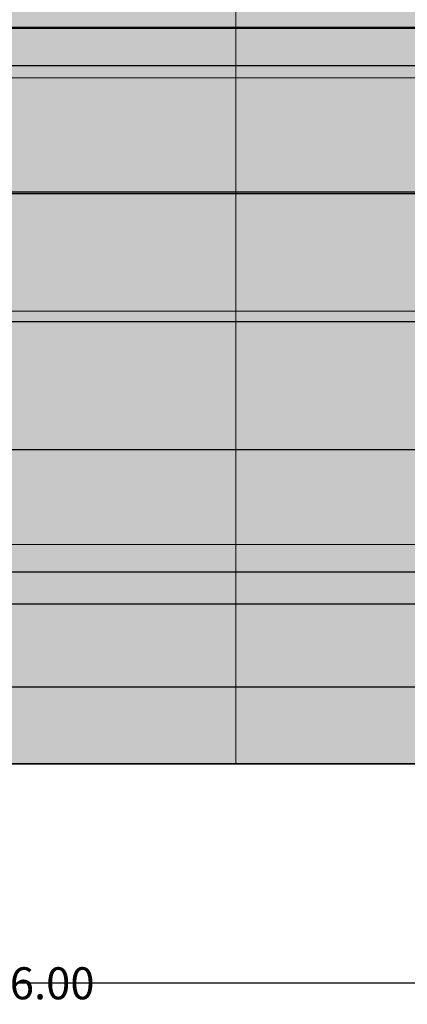
# Model space of a CAD drawing. Units: inches. Extents: x 148 to 1080, y 89 to 707.
# Tile 4 of 12: x 397 to 470, y 89 to 273. Entities that reach past the tile are written whole.
import ezdxf

# ---------------------------------------------------------------- set-up
doc = ezdxf.new("R2010")
doc.units = ezdxf.units.IN
doc.header["$MEASUREMENT"] = 0
for name, color, linetype, lineweight in [('A-ANNO-DIMS', 2, 'Continuous', 18), ('A-ELEV', 7, 'Continuous', 35), ('A-ELEV-PATT', 8, 'Continuous', 13)]:
    doc.layers.add(name, color=color, linetype=linetype, lineweight=lineweight)
doc.styles.get("Standard").update_dxf_attribs({"font": 'arial.ttf'})
doc.dimstyles.get("Standard").update_dxf_attribs({"dimtxt": 6, "dimasz": 0.18, "dimexe": 0.18, "dimexo": 0.0625, "dimgap": 0.09, "dimtad": 0, "dimtih": 1, "dimtoh": 1, "dimdec": 0, "dimzin": 0, "dimdsep": 46, "dimlunit": 3, "dimtxsty": 'Standard', "dimcen": 0.09, "dimadec": 0, "dimazin": 0, "dimtfac": 1, "dimtdec": 0, "dimtofl": 0, "dimtmove": 0, "dimatfit": 3, "dimfxl": 1, "dimtolj": 1, "dimtzin": 0, "dimarcsym": 0})

# ---------------------------------------------------------------- blocks, each defined once
blk = doc.blocks.new('*D2')
at = {"layer": 'A-ANNO-DIMS', "color": 0, "lineweight": -2, "transparency": 16777216}
for p, q in [((251.02, 133.88), (251.02, 92.62)), ((527.02, 133.88), (527.02, 92.62)), ((251.2, 92.8), (382.25, 92.8)), ((526.84, 92.8), (395.79, 92.8))]:
    blk.add_line(p, q, dxfattribs=at)
at = {"layer": 'A-ANNO-DIMS', "color": 0, "transparency": 16777216}
for points in [[(251.2, 92.83), (251.2, 92.77), (251.02, 92.8)], [(526.84, 92.83), (526.84, 92.77), (527.02, 92.8)]]:
    blk.add_solid(points, dxfattribs=at)
at = {"layer": 'Defpoints', "color": 0, "transparency": 16777216}
for p in [(251.02, 133.95), (527.02, 133.95), (527.02, 92.8)]:
    blk.add_point(p, dxfattribs=at)
at = {"layer": 'A-ANNO-DIMS', "color": 0, "transparency": 16777216, "insert": (389.02, 92.8), "char_height": 6, "attachment_point": 5}
blk.add_mtext('\\A1;276', dxfattribs=at)
blk = doc.blocks.new('*D32')
at = {"layer": 'A-ANNO-DIMS', "color": 0, "lineweight": -2, "transparency": 16777216}
for p, q in [((587, 271.77), (160.42, 271.77)), ((160.6, 271.59), (160.6, 213.18)), ((160.6, 148.46), (160.6, 206.87)), ((587, 148.28), (160.42, 148.28))]:
    blk.add_line(p, q, dxfattribs=at)
at = {"layer": 'A-ANNO-DIMS', "color": 0, "transparency": 16777216}
for points in [[(160.57, 271.59), (160.63, 271.59), (160.6, 271.77)], [(160.57, 148.46), (160.63, 148.46), (160.6, 148.28)]]:
    blk.add_solid(points, dxfattribs=at)
at = {"layer": 'Defpoints', "color": 0, "transparency": 16777216}
for p in [(160.6, 271.77), (587.06, 271.77), (587.06, 148.28)]:
    blk.add_point(p, dxfattribs=at)
at = {"layer": 'A-ANNO-DIMS', "color": 0, "transparency": 16777216, "insert": (160.6, 210.03), "char_height": 6, "attachment_point": 5}
blk.add_mtext('\\A1;123.5', dxfattribs=at)
blk = doc.blocks.new('*D34')
at = {"layer": 'A-ANNO-DIMS', "color": 0, "lineweight": -2, "transparency": 16777216}
for p, q in [((574.96, 283.95), (160.42, 283.95)), ((160.6, 283.77), (160.6, 212.1)), ((160.6, 134.13), (160.6, 205.79)), ((574.96, 133.95), (160.42, 133.95))]:
    blk.add_line(p, q, dxfattribs=at)
at = {"layer": 'A-ANNO-DIMS', "color": 0, "transparency": 16777216}
for points in [[(160.57, 283.77), (160.63, 283.77), (160.6, 283.95)], [(160.57, 134.13), (160.63, 134.13), (160.6, 133.95)]]:
    blk.add_solid(points, dxfattribs=at)
at = {"layer": 'Defpoints', "color": 0, "transparency": 16777216}
for p in [(575.02, 283.95), (160.6, 133.95), (575.02, 133.95)]:
    blk.add_point(p, dxfattribs=at)
at = {"layer": 'A-ANNO-DIMS', "color": 0, "transparency": 16777216, "insert": (160.6, 208.95), "char_height": 6, "attachment_point": 5}
blk.add_mtext('\\A1;150', dxfattribs=at)
blk = doc.blocks.new('*D38')
at = {"layer": 'A-ANNO-DIMS', "color": 0, "lineweight": -2, "transparency": 16777216}
for p, q in [((934.89, 271.95), (160.42, 271.95)), ((160.6, 271.77), (160.6, 206.1)), ((160.6, 134.13), (160.6, 199.79)), ((934.89, 133.95), (160.42, 133.95))]:
    blk.add_line(p, q, dxfattribs=at)
at = {"layer": 'A-ANNO-DIMS', "color": 0, "transparency": 16777216}
for points in [[(160.57, 271.77), (160.63, 271.77), (160.6, 271.95)], [(160.57, 134.13), (160.63, 134.13), (160.6, 133.95)]]:
    blk.add_solid(points, dxfattribs=at)
at = {"layer": 'Defpoints', "color": 0, "transparency": 16777216}
for p in [(934.95, 271.95), (160.6, 133.95), (934.95, 133.95)]:
    blk.add_point(p, dxfattribs=at)
at = {"layer": 'A-ANNO-DIMS', "color": 0, "transparency": 16777216, "insert": (160.6, 202.95), "char_height": 6, "attachment_point": 5}
blk.add_mtext('\\A1;138', dxfattribs=at)
blk = doc.blocks.new('*D43')
at = {"layer": 'A-ANNO-DIMS', "color": 0, "lineweight": -2, "transparency": 16777216}
for p, q in [((765.88, 241.1), (160.42, 241.1)), ((160.6, 240.92), (160.6, 190.68)), ((160.6, 134.13), (160.6, 184.37)), ((776.65, 133.95), (160.42, 133.95))]:
    blk.add_line(p, q, dxfattribs=at)
at = {"layer": 'A-ANNO-DIMS', "color": 0, "transparency": 16777216}
for points in [[(160.57, 240.92), (160.63, 240.92), (160.6, 241.1)], [(160.57, 134.13), (160.63, 134.13), (160.6, 133.95)]]:
    blk.add_solid(points, dxfattribs=at)
at = {"layer": 'Defpoints', "color": 0, "transparency": 16777216}
for p in [(765.95, 241.1), (160.6, 133.95), (776.71, 133.95)]:
    blk.add_point(p, dxfattribs=at)
at = {"layer": 'A-ANNO-DIMS', "color": 0, "transparency": 16777216, "insert": (160.6, 187.52), "char_height": 6, "attachment_point": 5}
blk.add_mtext('\\A1;107.15', dxfattribs=at)
blk = doc.blocks.new('*D70')
at = {"layer": 'A-ANNO-DIMS', "color": 0, "lineweight": -2, "transparency": 16777216}
for p, q in [((389.02, 169.88), (389.02, 92.62)), ((395.02, 163.88), (395.02, 92.62)), ((389.2, 92.8), (394.84, 92.8)), ((395.02, 92.8), (395.2, 92.8))]:
    blk.add_line(p, q, dxfattribs=at)
at = {"layer": 'A-ANNO-DIMS', "color": 0, "transparency": 16777216}
for points in [[(389.2, 92.83), (389.2, 92.77), (389.02, 92.8)], [(394.84, 92.83), (394.84, 92.77), (395.02, 92.8)]]:
    blk.add_solid(points, dxfattribs=at)
at = {"layer": 'Defpoints', "color": 0, "transparency": 16777216}
for p in [(389.02, 169.95), (395.02, 163.95), (395.02, 92.8)]:
    blk.add_point(p, dxfattribs=at)
at = {"layer": 'A-ANNO-DIMS', "color": 0, "transparency": 16777216, "insert": (403.09, 92.8), "char_height": 6, "attachment_point": 5}
blk.add_mtext('\\A1;6.00', dxfattribs=at)
blk = doc.blocks.new('*D71')
at = {"layer": 'A-ANNO-DIMS', "color": 0, "lineweight": -2, "transparency": 16777216}
for p, q in [((389.08, 169.95), (1064.5, 169.95)), ((1064.32, 169.95), (1064.32, 170.13)), ((1064.32, 170.13), (1064.5, 170.13)), ((1064.32, 164.13), (1064.32, 169.77)), ((395.08, 163.95), (1064.5, 163.95))]:
    blk.add_line(p, q, dxfattribs=at)
at = {"layer": 'A-ANNO-DIMS', "color": 0, "transparency": 16777216}
for points in [[(1064.29, 169.77), (1064.35, 169.77), (1064.32, 169.95)], [(1064.29, 164.13), (1064.35, 164.13), (1064.32, 163.95)]]:
    blk.add_solid(points, dxfattribs=at)
at = {"layer": 'Defpoints', "color": 0, "transparency": 16777216}
for p in [(389.02, 169.95), (1064.32, 169.95), (395.02, 163.95)]:
    blk.add_point(p, dxfattribs=at)
at = {"layer": 'A-ANNO-DIMS', "color": 0, "transparency": 16777216, "insert": (1072.39, 170.13), "char_height": 6, "attachment_point": 5}
blk.add_mtext('\\A1;6.00', dxfattribs=at)
blk = doc.blocks.new('*D72')
at = {"layer": 'A-ANNO-DIMS', "color": 0, "lineweight": -2, "transparency": 16777216}
for p, q in [((389.08, 192.87), (1064.5, 192.87)), ((1064.32, 192.69), (1064.32, 184.56)), ((1064.32, 170.13), (1064.32, 178.26)), ((389.08, 169.95), (1064.5, 169.95))]:
    blk.add_line(p, q, dxfattribs=at)
at = {"layer": 'A-ANNO-DIMS', "color": 0, "transparency": 16777216}
for points in [[(1064.29, 192.69), (1064.35, 192.69), (1064.32, 192.87)], [(1064.29, 170.13), (1064.35, 170.13), (1064.32, 169.95)]]:
    blk.add_solid(points, dxfattribs=at)
at = {"layer": 'Defpoints', "color": 0, "transparency": 16777216}
for p in [(389.02, 192.87), (1064.32, 192.87), (389.02, 169.95)]:
    blk.add_point(p, dxfattribs=at)
at = {"layer": 'A-ANNO-DIMS', "color": 0, "transparency": 16777216, "insert": (1064.32, 181.41), "char_height": 6, "attachment_point": 5}
blk.add_mtext('\\A1;22.92', dxfattribs=at)
blk = doc.blocks.new('*D73')
at = {"layer": 'A-ANNO-DIMS', "color": 0, "lineweight": -2, "transparency": 16777216}
for p, q in [((389.08, 216.87), (1064.5, 216.87)), ((1064.32, 216.69), (1064.32, 208.02)), ((1064.32, 193.05), (1064.32, 201.72)), ((389.08, 192.87), (1064.5, 192.87))]:
    blk.add_line(p, q, dxfattribs=at)
at = {"layer": 'A-ANNO-DIMS', "color": 0, "transparency": 16777216}
for points in [[(1064.29, 216.69), (1064.35, 216.69), (1064.32, 216.87)], [(1064.29, 193.05), (1064.35, 193.05), (1064.32, 192.87)]]:
    blk.add_solid(points, dxfattribs=at)
at = {"layer": 'Defpoints', "color": 0, "transparency": 16777216}
for p in [(389.02, 216.87), (1064.32, 216.87), (389.02, 192.87)]:
    blk.add_point(p, dxfattribs=at)
at = {"layer": 'A-ANNO-DIMS', "color": 0, "transparency": 16777216, "insert": (1064.32, 204.87), "char_height": 6, "attachment_point": 5}
blk.add_mtext('\\A1;24.00', dxfattribs=at)
blk = doc.blocks.new('*D74')
at = {"layer": 'A-ANNO-DIMS', "color": 0, "lineweight": -2, "transparency": 16777216}
for p, q in [((389.08, 240.87), (1064.5, 240.87)), ((1064.32, 240.69), (1064.32, 232.02)), ((1064.32, 217.05), (1064.32, 225.72)), ((389.08, 216.87), (1064.5, 216.87))]:
    blk.add_line(p, q, dxfattribs=at)
at = {"layer": 'A-ANNO-DIMS', "color": 0, "transparency": 16777216}
for points in [[(1064.29, 240.69), (1064.35, 240.69), (1064.32, 240.87)], [(1064.29, 217.05), (1064.35, 217.05), (1064.32, 216.87)]]:
    blk.add_solid(points, dxfattribs=at)
at = {"layer": 'Defpoints', "color": 0, "transparency": 16777216}
for p in [(389.02, 240.87), (1064.32, 240.87), (389.02, 216.87)]:
    blk.add_point(p, dxfattribs=at)
at = {"layer": 'A-ANNO-DIMS', "color": 0, "transparency": 16777216, "insert": (1064.32, 228.87), "char_height": 6, "attachment_point": 5}
blk.add_mtext('\\A1;24.00', dxfattribs=at)
blk = doc.blocks.new('*D75')
at = {"layer": 'A-ANNO-DIMS', "color": 0, "lineweight": -2, "transparency": 16777216}
for p, q in [((389.08, 264.87), (1064.5, 264.87)), ((1064.32, 264.69), (1064.32, 256.02)), ((1064.32, 241.05), (1064.32, 249.72)), ((389.08, 240.87), (1064.5, 240.87))]:
    blk.add_line(p, q, dxfattribs=at)
at = {"layer": 'A-ANNO-DIMS', "color": 0, "transparency": 16777216}
for points in [[(1064.29, 264.69), (1064.35, 264.69), (1064.32, 264.87)], [(1064.29, 241.05), (1064.35, 241.05), (1064.32, 240.87)]]:
    blk.add_solid(points, dxfattribs=at)
at = {"layer": 'Defpoints', "color": 0, "transparency": 16777216}
for p in [(389.02, 264.87), (1064.32, 264.87), (389.02, 240.87)]:
    blk.add_point(p, dxfattribs=at)
at = {"layer": 'A-ANNO-DIMS', "color": 0, "transparency": 16777216, "insert": (1064.32, 252.87), "char_height": 6, "attachment_point": 5}
blk.add_mtext('\\A1;24.00', dxfattribs=at)
blk = doc.blocks.new('*D76')
at = {"layer": 'A-ANNO-DIMS', "color": 0, "lineweight": -2, "transparency": 16777216}
for p, q in [((389.08, 300.95), (1064.5, 300.95)), ((1064.32, 300.77), (1064.32, 286.06)), ((1064.32, 265.05), (1064.32, 279.75)), ((389.08, 264.87), (1064.5, 264.87))]:
    blk.add_line(p, q, dxfattribs=at)
at = {"layer": 'A-ANNO-DIMS', "color": 0, "transparency": 16777216}
for points in [[(1064.29, 300.77), (1064.35, 300.77), (1064.32, 300.95)], [(1064.29, 265.05), (1064.35, 265.05), (1064.32, 264.87)]]:
    blk.add_solid(points, dxfattribs=at)
at = {"layer": 'Defpoints', "color": 0, "transparency": 16777216}
for p in [(389.02, 300.95), (1064.32, 300.95), (389.02, 264.87)]:
    blk.add_point(p, dxfattribs=at)
at = {"layer": 'A-ANNO-DIMS', "color": 0, "transparency": 16777216, "insert": (1064.32, 282.91), "char_height": 6, "attachment_point": 5}
blk.add_mtext('\\A1;36.08', dxfattribs=at)
blk = doc.blocks.new('*D89')
at = {"layer": 'A-ANNO-DIMS', "color": 0, "lineweight": -2, "transparency": 16777216}
for p, q in [((389.02, 400.88), (389.02, 92.62)), ((395.02, 400.88), (395.02, 92.62)), ((389.2, 92.8), (394.84, 92.8)), ((395.02, 92.8), (395.2, 92.8))]:
    blk.add_line(p, q, dxfattribs=at)
at = {"layer": 'A-ANNO-DIMS', "color": 0, "transparency": 16777216}
for points in [[(389.2, 92.83), (389.2, 92.77), (389.02, 92.8)], [(394.84, 92.83), (394.84, 92.77), (395.02, 92.8)]]:
    blk.add_solid(points, dxfattribs=at)
at = {"layer": 'Defpoints', "color": 0, "transparency": 16777216}
for p in [(389.02, 400.95), (395.02, 400.95), (395.02, 92.8)]:
    blk.add_point(p, dxfattribs=at)
at = {"layer": 'A-ANNO-DIMS', "color": 0, "transparency": 16777216, "insert": (403.09, 92.8), "char_height": 6, "attachment_point": 5}
blk.add_mtext('\\A1;6.00', dxfattribs=at)
blk = doc.blocks.new('*D102')
at = {"layer": 'A-ANNO-DIMS', "color": 0, "lineweight": -2, "transparency": 16777216}
for p, q in [((742.96, 271.95), (160.42, 271.95)), ((160.6, 271.77), (160.6, 259.68)), ((160.6, 241.28), (160.6, 253.37)), ((765.88, 241.1), (160.42, 241.1))]:
    blk.add_line(p, q, dxfattribs=at)
at = {"layer": 'A-ANNO-DIMS', "color": 0, "transparency": 16777216}
for points in [[(160.57, 271.77), (160.63, 271.77), (160.6, 271.95)], [(160.57, 241.28), (160.63, 241.28), (160.6, 241.1)]]:
    blk.add_solid(points, dxfattribs=at)
at = {"layer": 'Defpoints', "color": 0, "transparency": 16777216}
for p in [(160.6, 271.95), (743.02, 271.95), (765.95, 241.1)]:
    blk.add_point(p, dxfattribs=at)
at = {"layer": 'A-ANNO-DIMS', "color": 0, "transparency": 16777216, "insert": (160.6, 256.52), "char_height": 6, "attachment_point": 5}
blk.add_mtext('\\A1;30.85', dxfattribs=at)

msp = doc.modelspace()

# ---------------------------------------------------------------- hatches: boundary and pattern name
at = {"layer": 'A-ELEV-PATT'}
h = msp.add_hatch(color=256, dxfattribs=at)
h.dxf.hatch_style = 1
h.paths.add_polyline_path([(527.0199, 349.9474), (395.0199, 349.9474), (395.0199, 271.2774), (527.0199, 272.3839)])
h.paths.add_polyline_path([(275.0199, 349.9474), (251.0199, 349.9474), (251.0199, 270.0704), (275.0199, 270.2716)])
h.paths.add_polyline_path([(743.0199, 337.9474), (734.0628, 337.9474), (719.0199, 326.3632), (719.0199, 277.9474), (743.0199, 277.9474)])
h.paths.add_polyline_path([(743.0199, 277.9474), (719.0199, 277.9474), (719.0199, 133.9474), (743.0199, 133.9474)])
h.paths.add_polyline_path([(734.0628, 337.9474), (719.0199, 337.9474), (719.0199, 326.3632)])
h = msp.add_hatch(dxfattribs=at)
h.set_pattern_fill('ANSI37', color=256, scale=350, angle=135)
h.paths.add_polyline_path([(527.0199, 349.9474), (395.0199, 349.9474), (395.0199, 163.9474), (275.0199, 163.9474), (275.0199, 349.9474), (251.0199, 349.9474), (251.0199, 133.9474), (527.0199, 133.9474)])
h = msp.add_hatch(color=256, dxfattribs=at)
h.dxf.hatch_style = 1
h.paths.add_polyline_path([(527.0199, 272.3839), (395.0199, 271.2774), (395.0199, 163.9474), (275.0199, 163.9474), (275.0199, 270.2716), (251.0199, 270.0704), (251.0199, 133.9474), (527.0199, 133.9474)])
h.paths.add_polyline_path([(1006.9492, 337.9474), (946.9492, 337.9474), (946.9492, 277.9474), (1006.9492, 277.9474)])
h.paths.add_polyline_path([(1006.9492, 277.9474), (946.9492, 277.9474), (946.9492, 133.9474), (1006.9492, 133.9474)])
h.paths.add_polyline_path([(946.9492, 337.9474), (743.0199, 337.9474), (743.0199, 277.9474), (946.9492, 277.9474)])

# ---------------------------------------------------------------- linework, layer by layer
at = {"layer": 'A-ELEV'}
msp.add_line((201.7492, 133.9474), (1023.175, 133.9474), dxfattribs=at)

# ---------------------------------------------------------------- dimensions: what is measured, and where the dimension line sits
at = {"layer": 'A-ANNO-DIMS'}
for base, p1, p2, override, picture, middle in [((395.0199, 92.7974), (389.0199, 400.9474), (395.0199, 400.9474), {"dimdec": 2, "dimlfac": 1, "dimrnd": 0, "dimzin": 0, "dimdsep": 46, "dimlunit": 2}, '*D89', (403.0886, 92.7974)), ((395.0199, 92.7974), (389.0199, 169.9474), (395.0199, 163.9474), {"dimdec": 2, "dimlfac": 1, "dimrnd": 0, "dimzin": 0, "dimdsep": 46, "dimlunit": 2}, '*D70', (403.0886, 92.7974)), ((527.0199, 92.7974), (251.0199, 133.9474), (527.0199, 133.9474), {"dimdec": 0, "dimlfac": 1, "dimrnd": 0, "dimzin": 0, "dimdsep": 46, "dimlunit": 2}, '*D2', (389.0199, 92.7974))]:
    dim = msp.add_linear_dim(base=base, p1=p1, p2=p2, dimstyle='Standard', override=override, dxfattribs=at)
    dim.commit()
    dim.dimension.update_dxf_attribs({"geometry": picture, "text_midpoint": middle})
for base, p1, p2, override, picture, middle in [((1064.325, 300.9474), (389.0199, 264.8696), (389.0199, 300.9474), {"dimdec": 2, "dimlfac": 1, "dimrnd": 0, "dimzin": 0, "dimdsep": 46, "dimlunit": 2}, '*D76', (1064.325, 282.9085)), ((160.5992, 133.9474), (575.0199, 283.9474), (575.0199, 133.9474), {"dimdec": 0, "dimlfac": 1, "dimrnd": 0, "dimzin": 0, "dimdsep": 46, "dimlunit": 2}, '*D34', (160.5992, 208.9474)), ((160.5992, 271.9474), (765.9474, 241.0996), (743.0199, 271.9474), {"dimdec": 2, "dimlfac": 1, "dimrnd": 0, "dimzin": 0, "dimdsep": 46, "dimlunit": 2}, '*D102', (160.5992, 256.5235)), ((160.5992, 271.7747), (587.0631, 148.2809), (587.0631, 271.7747), {"dimdec": 1, "dimlfac": 1, "dimrnd": 0, "dimzin": 0, "dimdsep": 46, "dimlunit": 2}, '*D32', (160.5992, 210.0278)), ((160.5992, 133.9474), (934.9492, 271.9474), (934.9492, 133.9474), {"dimdec": 0, "dimlfac": 1, "dimrnd": 0, "dimzin": 0, "dimdsep": 46, "dimlunit": 2}, '*D38', (160.5992, 202.9474)), ((1064.325, 264.8696), (389.0199, 240.8696), (389.0199, 264.8696), {"dimdec": 2, "dimlfac": 1, "dimrnd": 0, "dimzin": 0, "dimdsep": 46, "dimlunit": 2}, '*D75', (1064.325, 252.8696)), ((160.5992, 133.9474), (765.9474, 241.0996), (776.713, 133.9474), {"dimdec": 2, "dimlfac": 1, "dimrnd": 0, "dimzin": 0, "dimdsep": 46, "dimlunit": 2}, '*D43', (160.5992, 187.5235)), ((1064.325, 240.8696), (389.0199, 216.8696), (389.0199, 240.8696), {"dimdec": 2, "dimlfac": 1, "dimrnd": 0, "dimzin": 0, "dimdsep": 46, "dimlunit": 2}, '*D74', (1064.325, 228.8696)), ((1064.325, 216.8696), (389.0199, 192.8696), (389.0199, 216.8696), {"dimdec": 2, "dimlfac": 1, "dimrnd": 0, "dimzin": 0, "dimdsep": 46, "dimlunit": 2}, '*D73', (1064.325, 204.8696)), ((1064.325, 192.8696), (389.0199, 169.9474), (389.0199, 192.8696), {"dimdec": 2, "dimlfac": 1, "dimrnd": 0, "dimzin": 0, "dimdsep": 46, "dimlunit": 2}, '*D72', (1064.325, 181.4085)), ((1064.325, 169.9474), (395.0199, 163.9474), (389.0199, 169.9474), {"dimdec": 2, "dimlfac": 1, "dimrnd": 0, "dimzin": 0, "dimdsep": 46, "dimlunit": 2}, '*D71', (1072.3937, 170.1274))]:
    dim = msp.add_linear_dim(base=base, p1=p1, p2=p2, angle=90, dimstyle='Standard', override=override, dxfattribs=at)
    dim.commit()
    dim.dimension.update_dxf_attribs({"geometry": picture, "text_midpoint": middle})

doc.saveas('drawing.dxf')
